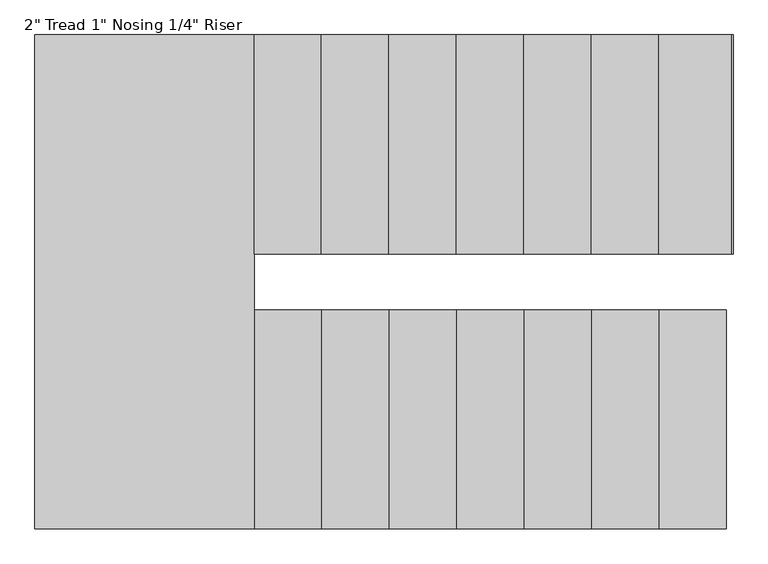
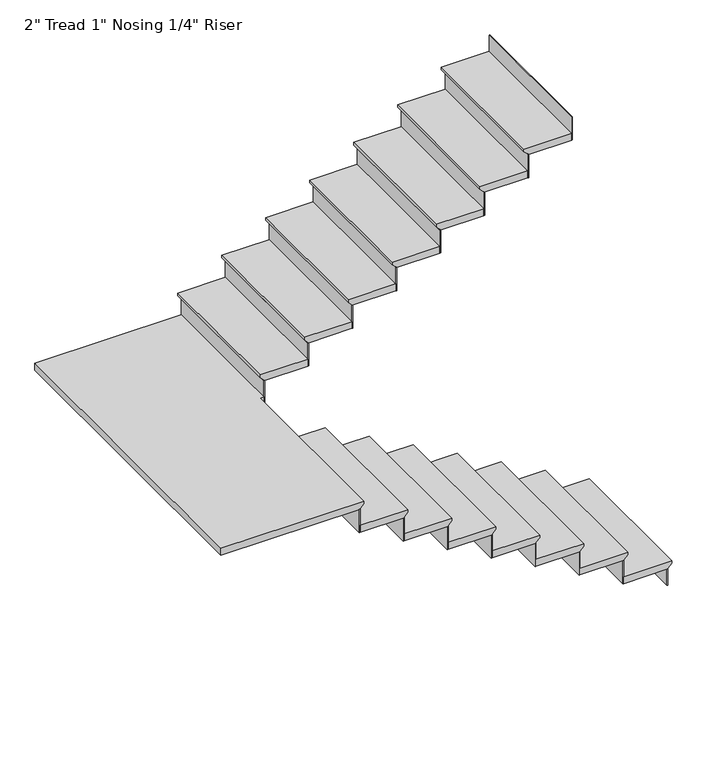
"""IFC4 building model written with IfcOpenShell, lengths in millimetres: stair flight geometry."""

from ifc_helpers import new_model, si_unit, origin, place, context, project, spatial, faceted_brep, source, transform, mapped, element, save


def stair_flight_128b20ea(model_context):
    return source(origin(), model_context, "Body", "Brep", [
        faceted_brep([(-11636.5023867, -1766.1499863, 3807.8833333), (-11636.5023867, -1766.1499863, 3826.9333333), (-11636.5023867, -2756.7499863, 3826.9333333), (-11636.5023867, -2756.7499863, 3807.8833333), (-11661.9023867, -1766.1499863, 3782.4833333), (-11661.9023867, -2756.7499863, 3782.4833333), (-11966.7023867, -1766.1499863, 3826.9333333), (-11966.7023867, -2756.7499863, 3826.9333333), (-11661.9023867, -2756.7499863, 3776.1333333), (-11966.7023867, -2756.7499863, 3776.1333333), (-11966.7023867, -1766.1499863, 3776.1333333), (-11661.9023867, -1766.1499863, 3776.1333333)], [[[0, 1, 2, 3]], [[4, 0, 3, 5]], [[2, 1, 6, 7]], [[8, 9, 10, 11]], [[2, 7, 9, 8, 5, 3]], [[8, 11, 4, 5]], [[6, 1, 0, 4, 11, 10]], [[7, 6, 10, 9]]]),
        faceted_brep([(-11661.9023867, -1766.1499863, 3776.1333333), (-11661.9023867, -1766.1499863, 3657.6), (-11668.2523867, -1766.1499863, 3657.6), (-11668.2523867, -1766.1499863, 3776.1333333), (-11661.9023867, -2756.7499863, 3776.1333333), (-11668.2523867, -2756.7499863, 3776.1333333), (-11668.2523867, -2756.7499863, 3657.6), (-11661.9023867, -2756.7499863, 3657.6)], [[[0, 1, 2, 3]], [[4, 5, 6, 7]], [[1, 0, 4, 7]], [[2, 1, 7, 6]], [[3, 2, 6, 5]], [[0, 3, 5, 4]]]),
        faceted_brep([(-11966.7023867, -1766.1499863, 3945.4666667), (-11966.7023867, -1766.1499863, 3776.1333333), (-11973.0523867, -1766.1499863, 3776.1333333), (-11973.0523867, -1766.1499863, 3945.4666667), (-11966.7023867, -2756.7499863, 3945.4666667), (-11973.0523867, -2756.7499863, 3945.4666667), (-11973.0523867, -2756.7499863, 3776.1333333), (-11966.7023867, -2756.7499863, 3776.1333333)], [[[0, 1, 2, 3]], [[4, 5, 6, 7]], [[1, 0, 4, 7]], [[2, 1, 7, 6]], [[3, 2, 6, 5]], [[0, 3, 5, 4]]]),
        faceted_brep([(-11941.3023867, -2756.7499863, 3996.2666667), (-11941.3023867, -1766.1499863, 3996.2666667), (-12271.5023867, -1766.1499863, 3996.2666667), (-12271.5023867, -2756.7499863, 3996.2666667), (-11966.7023867, -2756.7499863, 3945.4666667), (-12271.5023867, -2756.7499863, 3945.4666667), (-12271.5023867, -1766.1499863, 3945.4666667), (-11966.7023867, -1766.1499863, 3945.4666667), (-11966.7023867, -2756.7499863, 3951.8166667), (-11941.3023867, -2756.7499863, 3977.2166667), (-11966.7023867, -1766.1499863, 3951.8166667), (-11941.3023867, -1766.1499863, 3977.2166667)], [[[0, 1, 2, 3]], [[4, 5, 6, 7]], [[0, 3, 5, 4, 8, 9]], [[4, 7, 10, 8]], [[2, 1, 11, 10, 7, 6]], [[3, 2, 6, 5]], [[11, 1, 0, 9]], [[10, 11, 9, 8]]]),
        faceted_brep([(-12271.5023867, -1766.1499863, 4114.8), (-12271.5023867, -1766.1499863, 3945.4666667), (-12277.8523867, -1766.1499863, 3945.4666667), (-12277.8523867, -1766.1499863, 4114.8), (-12271.5023867, -2756.7499863, 4114.8), (-12277.8523867, -2756.7499863, 4114.8), (-12277.8523867, -2756.7499863, 3945.4666667), (-12271.5023867, -2756.7499863, 3945.4666667)], [[[0, 1, 2, 3]], [[4, 5, 6, 7]], [[1, 0, 4, 7]], [[2, 1, 7, 6]], [[3, 2, 6, 5]], [[0, 3, 5, 4]]]),
        faceted_brep([(-12246.1023867, -2756.7499863, 4165.6), (-12246.1023867, -1766.1499863, 4165.6), (-12576.3023867, -1766.1499863, 4165.6), (-12576.3023867, -2756.7499863, 4165.6), (-12271.5023867, -2756.7499863, 4114.8), (-12576.3023867, -2756.7499863, 4114.8), (-12576.3023867, -1766.1499863, 4114.8), (-12271.5023867, -1766.1499863, 4114.8), (-12271.5023867, -2756.7499863, 4121.15), (-12246.1023867, -2756.7499863, 4146.55), (-12271.5023867, -1766.1499863, 4121.15), (-12246.1023867, -1766.1499863, 4146.55)], [[[0, 1, 2, 3]], [[4, 5, 6, 7]], [[0, 3, 5, 4, 8, 9]], [[4, 7, 10, 8]], [[2, 1, 11, 10, 7, 6]], [[3, 2, 6, 5]], [[11, 1, 0, 9]], [[10, 11, 9, 8]]]),
        faceted_brep([(-12576.3023867, -1766.1499863, 4284.1333333), (-12576.3023867, -1766.1499863, 4114.8), (-12582.6523867, -1766.1499863, 4114.8), (-12582.6523867, -1766.1499863, 4284.1333333), (-12576.3023867, -2756.7499863, 4284.1333333), (-12582.6523867, -2756.7499863, 4284.1333333), (-12582.6523867, -2756.7499863, 4114.8), (-12576.3023867, -2756.7499863, 4114.8)], [[[0, 1, 2, 3]], [[4, 5, 6, 7]], [[1, 0, 4, 7]], [[2, 1, 7, 6]], [[3, 2, 6, 5]], [[0, 3, 5, 4]]]),
        faceted_brep([(-12550.9023867, -2756.7499863, 4334.9333333), (-12550.9023867, -1766.1499863, 4334.9333333), (-12881.1023867, -1766.1499863, 4334.9333333), (-12881.1023867, -2756.7499863, 4334.9333333), (-12576.3023867, -2756.7499863, 4284.1333333), (-12881.1023867, -2756.7499863, 4284.1333333), (-12881.1023867, -1766.1499863, 4284.1333333), (-12576.3023867, -1766.1499863, 4284.1333333), (-12576.3023867, -2756.7499863, 4290.4833333), (-12550.9023867, -2756.7499863, 4315.8833333), (-12576.3023867, -1766.1499863, 4290.4833333), (-12550.9023867, -1766.1499863, 4315.8833333)], [[[0, 1, 2, 3]], [[4, 5, 6, 7]], [[0, 3, 5, 4, 8, 9]], [[4, 7, 10, 8]], [[2, 1, 11, 10, 7, 6]], [[3, 2, 6, 5]], [[11, 1, 0, 9]], [[10, 11, 9, 8]]]),
        faceted_brep([(-12881.1023867, -1766.1499863, 4453.4666667), (-12881.1023867, -1766.1499863, 4284.1333333), (-12887.4523867, -1766.1499863, 4284.1333333), (-12887.4523867, -1766.1499863, 4453.4666667), (-12881.1023867, -2756.7499863, 4453.4666667), (-12887.4523867, -2756.7499863, 4453.4666667), (-12887.4523867, -2756.7499863, 4284.1333333), (-12881.1023867, -2756.7499863, 4284.1333333)], [[[0, 1, 2, 3]], [[4, 5, 6, 7]], [[1, 0, 4, 7]], [[2, 1, 7, 6]], [[3, 2, 6, 5]], [[0, 3, 5, 4]]]),
        faceted_brep([(-12855.7023867, -2756.7499863, 4504.2666667), (-12855.7023867, -1766.1499863, 4504.2666667), (-13185.9023867, -1766.1499863, 4504.2666667), (-13185.9023867, -2756.7499863, 4504.2666667), (-12881.1023867, -2756.7499863, 4453.4666667), (-13185.9023867, -2756.7499863, 4453.4666667), (-13185.9023867, -1766.1499863, 4453.4666667), (-12881.1023867, -1766.1499863, 4453.4666667), (-12881.1023867, -2756.7499863, 4459.8166667), (-12855.7023867, -2756.7499863, 4485.2166667), (-12881.1023867, -1766.1499863, 4459.8166667), (-12855.7023867, -1766.1499863, 4485.2166667)], [[[0, 1, 2, 3]], [[4, 5, 6, 7]], [[0, 3, 5, 4, 8, 9]], [[4, 7, 10, 8]], [[2, 1, 11, 10, 7, 6]], [[3, 2, 6, 5]], [[11, 1, 0, 9]], [[10, 11, 9, 8]]]),
        faceted_brep([(-13185.9023867, -1766.1499863, 4622.8), (-13185.9023867, -1766.1499863, 4453.4666667), (-13192.2523867, -1766.1499863, 4453.4666667), (-13192.2523867, -1766.1499863, 4622.8), (-13185.9023867, -2756.7499863, 4622.8), (-13192.2523867, -2756.7499863, 4622.8), (-13192.2523867, -2756.7499863, 4453.4666667), (-13185.9023867, -2756.7499863, 4453.4666667)], [[[0, 1, 2, 3]], [[4, 5, 6, 7]], [[1, 0, 4, 7]], [[2, 1, 7, 6]], [[3, 2, 6, 5]], [[0, 3, 5, 4]]]),
        faceted_brep([(-13160.5023867, -2756.7499863, 4673.6), (-13160.5023867, -1766.1499863, 4673.6), (-13490.7023867, -1766.1499863, 4673.6), (-13490.7023867, -2756.7499863, 4673.6), (-13185.9023867, -2756.7499863, 4622.8), (-13490.7023867, -2756.7499863, 4622.8), (-13490.7023867, -1766.1499863, 4622.8), (-13185.9023867, -1766.1499863, 4622.8), (-13185.9023867, -2756.7499863, 4629.15), (-13160.5023867, -2756.7499863, 4654.55), (-13185.9023867, -1766.1499863, 4629.15), (-13160.5023867, -1766.1499863, 4654.55)], [[[0, 1, 2, 3]], [[4, 5, 6, 7]], [[0, 3, 5, 4, 8, 9]], [[4, 7, 10, 8]], [[2, 1, 11, 10, 7, 6]], [[3, 2, 6, 5]], [[11, 1, 0, 9]], [[10, 11, 9, 8]]]),
        faceted_brep([(-13490.7023867, -1766.1499863, 4792.1333333), (-13490.7023867, -1766.1499863, 4622.8), (-13497.0523867, -1766.1499863, 4622.8), (-13497.0523867, -1766.1499863, 4792.1333333), (-13490.7023867, -2756.7499863, 4792.1333333), (-13497.0523867, -2756.7499863, 4792.1333333), (-13497.0523867, -2756.7499863, 4622.8), (-13490.7023867, -2756.7499863, 4622.8)], [[[0, 1, 2, 3]], [[4, 5, 6, 7]], [[1, 0, 4, 7]], [[2, 1, 7, 6]], [[3, 2, 6, 5]], [[0, 3, 5, 4]]]),
        faceted_brep([(-13465.3023867, -2756.7499863, 4842.9333333), (-13465.3023867, -1766.1499863, 4842.9333333), (-13795.5023867, -1766.1499863, 4842.9333333), (-13795.5023867, -2756.7499863, 4842.9333333), (-13490.7023867, -2756.7499863, 4792.1333333), (-13795.5023867, -2756.7499863, 4792.1333333), (-13795.5023867, -1766.1499863, 4792.1333333), (-13490.7023867, -1766.1499863, 4792.1333333), (-13490.7023867, -2756.7499863, 4798.4833333), (-13465.3023867, -2756.7499863, 4823.8833333), (-13490.7023867, -1766.1499863, 4798.4833333), (-13465.3023867, -1766.1499863, 4823.8833333)], [[[0, 1, 2, 3]], [[4, 5, 6, 7]], [[0, 3, 5, 4, 8, 9]], [[4, 7, 10, 8]], [[2, 1, 11, 10, 7, 6]], [[3, 2, 6, 5]], [[11, 1, 0, 9]], [[10, 11, 9, 8]]]),
        faceted_brep([(-13795.5023867, -1766.1499863, 4961.4666667), (-13795.5023867, -1766.1499863, 4792.1333333), (-13801.8523867, -1766.1499863, 4792.1333333), (-13801.8523867, -1766.1499863, 4961.4666667), (-13795.5023867, -2756.7499863, 4961.4666667), (-13801.8523867, -2756.7499863, 4961.4666667), (-13801.8523867, -2756.7499863, 4792.1333333), (-13795.5023867, -2756.7499863, 4792.1333333)], [[[0, 1, 2, 3]], [[4, 5, 6, 7]], [[1, 0, 4, 7]], [[2, 1, 7, 6]], [[3, 2, 6, 5]], [[0, 3, 5, 4]]]),
        faceted_brep([(-13744.7023867, -521.5499863, 5012.2666667), (-14760.7023867, -521.5499863, 5012.2666667), (-14760.7023867, -2756.7499863, 5012.2666667), (-13770.1023867, -2756.7499863, 5012.2666667), (-13770.1023867, -1512.1499863, 5012.2666667), (-13744.7023867, -1512.1499863, 5012.2666667), (-14760.7023867, -521.5499863, 4961.4666667), (-13744.7023867, -521.5499863, 4961.4666667), (-13744.7023867, -1512.1499863, 4961.4666667), (-13770.1023867, -1512.1499863, 4961.4666667), (-13770.1023867, -1766.1499863, 4961.4666667), (-13795.5023867, -1766.1499863, 4961.4666667), (-13795.5023867, -2756.7499863, 4961.4666667), (-14760.7023867, -2756.7499863, 4961.4666667), (-13795.5023867, -2756.7499863, 4967.8166667), (-13770.1023867, -2756.7499863, 4993.2166667), (-13795.5023867, -1766.1499863, 4967.8166667), (-13770.1023867, -1766.1499863, 4993.2166667)], [[[0, 1, 2, 3, 4, 5]], [[6, 7, 8, 9, 10, 11, 12, 13]], [[1, 0, 7, 6]], [[2, 1, 6, 13]], [[3, 2, 13, 12, 14, 15]], [[12, 11, 16, 14]], [[11, 10, 17, 16]], [[4, 3, 15, 17, 10, 9]], [[5, 4, 9, 8]], [[0, 5, 8, 7]], [[15, 14, 16, 17]]]),
        faceted_brep([(-13744.7023867, -1512.1499863, 5130.8), (-13744.7023867, -1512.1499863, 4961.4666667), (-13738.3523867, -1512.1499863, 4961.4666667), (-13738.3523867, -1512.1499863, 5130.8), (-13744.7023867, -521.5499863, 5130.8), (-13738.3523867, -521.5499863, 5130.8), (-13738.3523867, -521.5499863, 4961.4666667), (-13744.7023867, -521.5499863, 4961.4666667)], [[[0, 1, 2, 3]], [[4, 5, 6, 7]], [[1, 0, 4, 7]], [[2, 1, 7, 6]], [[3, 2, 6, 5]], [[0, 3, 5, 4]]]),
        faceted_brep([(-13770.1023867, -521.5499863, 5181.6), (-13770.1023867, -1512.1499863, 5181.6), (-13439.9023867, -1512.1499863, 5181.6), (-13439.9023867, -521.5499863, 5181.6), (-13744.7023867, -521.5499863, 5130.8), (-13439.9023867, -521.5499863, 5130.8), (-13439.9023867, -1512.1499863, 5130.8), (-13744.7023867, -1512.1499863, 5130.8), (-13744.7023867, -521.5499863, 5137.15), (-13770.1023867, -521.5499863, 5162.55), (-13744.7023867, -1512.1499863, 5137.15), (-13770.1023867, -1512.1499863, 5162.55)], [[[0, 1, 2, 3]], [[4, 5, 6, 7]], [[0, 3, 5, 4, 8, 9]], [[4, 7, 10, 8]], [[2, 1, 11, 10, 7, 6]], [[3, 2, 6, 5]], [[11, 1, 0, 9]], [[10, 11, 9, 8]]]),
        faceted_brep([(-13439.9023867, -1512.1499863, 5300.1333333), (-13439.9023867, -1512.1499863, 5130.8), (-13433.5523867, -1512.1499863, 5130.8), (-13433.5523867, -1512.1499863, 5300.1333333), (-13439.9023867, -521.5499863, 5300.1333333), (-13433.5523867, -521.5499863, 5300.1333333), (-13433.5523867, -521.5499863, 5130.8), (-13439.9023867, -521.5499863, 5130.8)], [[[0, 1, 2, 3]], [[4, 5, 6, 7]], [[1, 0, 4, 7]], [[2, 1, 7, 6]], [[3, 2, 6, 5]], [[0, 3, 5, 4]]]),
        faceted_brep([(-13465.3023867, -521.5499863, 5350.9333333), (-13465.3023867, -1512.1499863, 5350.9333333), (-13135.1023867, -1512.1499863, 5350.9333333), (-13135.1023867, -521.5499863, 5350.9333333), (-13439.9023867, -521.5499863, 5300.1333333), (-13135.1023867, -521.5499863, 5300.1333333), (-13135.1023867, -1512.1499863, 5300.1333333), (-13439.9023867, -1512.1499863, 5300.1333333), (-13439.9023867, -521.5499863, 5306.4833333), (-13465.3023867, -521.5499863, 5331.8833333), (-13439.9023867, -1512.1499863, 5306.4833333), (-13465.3023867, -1512.1499863, 5331.8833333)], [[[0, 1, 2, 3]], [[4, 5, 6, 7]], [[0, 3, 5, 4, 8, 9]], [[4, 7, 10, 8]], [[2, 1, 11, 10, 7, 6]], [[3, 2, 6, 5]], [[11, 1, 0, 9]], [[10, 11, 9, 8]]]),
        faceted_brep([(-13135.1023867, -1512.1499863, 5469.4666667), (-13135.1023867, -1512.1499863, 5300.1333333), (-13128.7523867, -1512.1499863, 5300.1333333), (-13128.7523867, -1512.1499863, 5469.4666667), (-13135.1023867, -521.5499863, 5469.4666667), (-13128.7523867, -521.5499863, 5469.4666667), (-13128.7523867, -521.5499863, 5300.1333333), (-13135.1023867, -521.5499863, 5300.1333333)], [[[0, 1, 2, 3]], [[4, 5, 6, 7]], [[1, 0, 4, 7]], [[2, 1, 7, 6]], [[3, 2, 6, 5]], [[0, 3, 5, 4]]]),
        faceted_brep([(-13160.5023867, -521.5499863, 5520.2666667), (-13160.5023867, -1512.1499863, 5520.2666667), (-12830.3023867, -1512.1499863, 5520.2666667), (-12830.3023867, -521.5499863, 5520.2666667), (-13135.1023867, -521.5499863, 5469.4666667), (-12830.3023867, -521.5499863, 5469.4666667), (-12830.3023867, -1512.1499863, 5469.4666667), (-13135.1023867, -1512.1499863, 5469.4666667), (-13135.1023867, -521.5499863, 5475.8166667), (-13160.5023867, -521.5499863, 5501.2166667), (-13135.1023867, -1512.1499863, 5475.8166667), (-13160.5023867, -1512.1499863, 5501.2166667)], [[[0, 1, 2, 3]], [[4, 5, 6, 7]], [[0, 3, 5, 4, 8, 9]], [[4, 7, 10, 8]], [[2, 1, 11, 10, 7, 6]], [[3, 2, 6, 5]], [[11, 1, 0, 9]], [[10, 11, 9, 8]]]),
        faceted_brep([(-12830.3023867, -1512.1499863, 5638.8), (-12830.3023867, -1512.1499863, 5469.4666667), (-12823.9523867, -1512.1499863, 5469.4666667), (-12823.9523867, -1512.1499863, 5638.8), (-12830.3023867, -521.5499863, 5638.8), (-12823.9523867, -521.5499863, 5638.8), (-12823.9523867, -521.5499863, 5469.4666667), (-12830.3023867, -521.5499863, 5469.4666667)], [[[0, 1, 2, 3]], [[4, 5, 6, 7]], [[1, 0, 4, 7]], [[2, 1, 7, 6]], [[3, 2, 6, 5]], [[0, 3, 5, 4]]]),
        faceted_brep([(-12855.7023867, -521.5499863, 5689.6), (-12855.7023867, -1512.1499863, 5689.6), (-12525.5023867, -1512.1499863, 5689.6), (-12525.5023867, -521.5499863, 5689.6), (-12830.3023867, -521.5499863, 5638.8), (-12525.5023867, -521.5499863, 5638.8), (-12525.5023867, -1512.1499863, 5638.8), (-12830.3023867, -1512.1499863, 5638.8), (-12830.3023867, -521.5499863, 5645.15), (-12855.7023867, -521.5499863, 5670.55), (-12830.3023867, -1512.1499863, 5645.15), (-12855.7023867, -1512.1499863, 5670.55)], [[[0, 1, 2, 3]], [[4, 5, 6, 7]], [[0, 3, 5, 4, 8, 9]], [[4, 7, 10, 8]], [[2, 1, 11, 10, 7, 6]], [[3, 2, 6, 5]], [[11, 1, 0, 9]], [[10, 11, 9, 8]]]),
        faceted_brep([(-12525.5023867, -1512.1499863, 5808.1333333), (-12525.5023867, -1512.1499863, 5638.8), (-12519.1523867, -1512.1499863, 5638.8), (-12519.1523867, -1512.1499863, 5808.1333333), (-12525.5023867, -521.5499863, 5808.1333333), (-12519.1523867, -521.5499863, 5808.1333333), (-12519.1523867, -521.5499863, 5638.8), (-12525.5023867, -521.5499863, 5638.8)], [[[0, 1, 2, 3]], [[4, 5, 6, 7]], [[1, 0, 4, 7]], [[2, 1, 7, 6]], [[3, 2, 6, 5]], [[0, 3, 5, 4]]]),
        faceted_brep([(-12550.9023867, -521.5499863, 5858.9333333), (-12550.9023867, -1512.1499863, 5858.9333333), (-12220.7023867, -1512.1499863, 5858.9333333), (-12220.7023867, -521.5499863, 5858.9333333), (-12525.5023867, -521.5499863, 5808.1333333), (-12220.7023867, -521.5499863, 5808.1333333), (-12220.7023867, -1512.1499863, 5808.1333333), (-12525.5023867, -1512.1499863, 5808.1333333), (-12525.5023867, -521.5499863, 5814.4833333), (-12550.9023867, -521.5499863, 5839.8833333), (-12525.5023867, -1512.1499863, 5814.4833333), (-12550.9023867, -1512.1499863, 5839.8833333)], [[[0, 1, 2, 3]], [[4, 5, 6, 7]], [[0, 3, 5, 4, 8, 9]], [[4, 7, 10, 8]], [[2, 1, 11, 10, 7, 6]], [[3, 2, 6, 5]], [[11, 1, 0, 9]], [[10, 11, 9, 8]]]),
        faceted_brep([(-12220.7023867, -1512.1499863, 5977.4666667), (-12220.7023867, -1512.1499863, 5808.1333333), (-12214.3523867, -1512.1499863, 5808.1333333), (-12214.3523867, -1512.1499863, 5977.4666667), (-12220.7023867, -521.5499863, 5977.4666667), (-12214.3523867, -521.5499863, 5977.4666667), (-12214.3523867, -521.5499863, 5808.1333333), (-12220.7023867, -521.5499863, 5808.1333333)], [[[0, 1, 2, 3]], [[4, 5, 6, 7]], [[1, 0, 4, 7]], [[2, 1, 7, 6]], [[3, 2, 6, 5]], [[0, 3, 5, 4]]]),
        faceted_brep([(-12246.1023867, -521.5499863, 6028.2666667), (-12246.1023867, -1512.1499863, 6028.2666667), (-11915.9023867, -1512.1499863, 6028.2666667), (-11915.9023867, -521.5499863, 6028.2666667), (-12220.7023867, -521.5499863, 5977.4666667), (-11915.9023867, -521.5499863, 5977.4666667), (-11915.9023867, -1512.1499863, 5977.4666667), (-12220.7023867, -1512.1499863, 5977.4666667), (-12220.7023867, -521.5499863, 5983.8166667), (-12246.1023867, -521.5499863, 6009.2166667), (-12220.7023867, -1512.1499863, 5983.8166667), (-12246.1023867, -1512.1499863, 6009.2166667)], [[[0, 1, 2, 3]], [[4, 5, 6, 7]], [[0, 3, 5, 4, 8, 9]], [[4, 7, 10, 8]], [[2, 1, 11, 10, 7, 6]], [[3, 2, 6, 5]], [[11, 1, 0, 9]], [[10, 11, 9, 8]]]),
        faceted_brep([(-11915.9023867, -1512.1499863, 6146.8), (-11915.9023867, -1512.1499863, 5977.4666667), (-11909.5523867, -1512.1499863, 5977.4666667), (-11909.5523867, -1512.1499863, 6146.8), (-11915.9023867, -521.5499863, 6146.8), (-11909.5523867, -521.5499863, 6146.8), (-11909.5523867, -521.5499863, 5977.4666667), (-11915.9023867, -521.5499863, 5977.4666667)], [[[0, 1, 2, 3]], [[4, 5, 6, 7]], [[1, 0, 4, 7]], [[2, 1, 7, 6]], [[3, 2, 6, 5]], [[0, 3, 5, 4]]]),
        faceted_brep([(-11611.1023867, -1512.1499863, 6316.1333333), (-11611.1023867, -1512.1499863, 6146.8), (-11604.7523867, -1512.1499863, 6146.8), (-11604.7523867, -1512.1499863, 6316.1333333), (-11611.1023867, -521.5499863, 6316.1333333), (-11604.7523867, -521.5499863, 6316.1333333), (-11604.7523867, -521.5499863, 6146.8), (-11611.1023867, -521.5499863, 6146.8)], [[[0, 1, 2, 3]], [[4, 5, 6, 7]], [[1, 0, 4, 7]], [[2, 1, 7, 6]], [[3, 2, 6, 5]], [[0, 3, 5, 4]]]),
        faceted_brep([(-11941.3023867, -521.5499863, 6197.6), (-11941.3023867, -1512.1499863, 6197.6), (-11611.1023867, -1512.1499863, 6197.6), (-11611.1023867, -521.5499863, 6197.6), (-11915.9023867, -521.5499863, 6146.8), (-11611.1023867, -521.5499863, 6146.8), (-11611.1023867, -1512.1499863, 6146.8), (-11915.9023867, -1512.1499863, 6146.8), (-11915.9023867, -521.5499863, 6153.15), (-11941.3023867, -521.5499863, 6178.55), (-11915.9023867, -1512.1499863, 6153.15), (-11941.3023867, -1512.1499863, 6178.55)], [[[0, 1, 2, 3]], [[4, 5, 6, 7]], [[0, 3, 5, 4, 8, 9]], [[4, 7, 10, 8]], [[2, 1, 11, 10, 7, 6]], [[3, 2, 6, 5]], [[11, 1, 0, 9]], [[10, 11, 9, 8]]]),
    ])


if __name__ == "__main__":
    model = new_model("IFC4")
    model_context = context("Model", 3, world=origin())
    ifc_project = project(units=[si_unit("LENGTHUNIT", "METRE", prefix="MILLI")], contexts=[model_context])
    site = spatial("IfcSite", under=ifc_project)
    building = spatial("IfcBuilding", under=site)
    placement = place(None, origin())
    stair_flight_shape = stair_flight_128b20ea(model_context)
    element("IfcStairFlight", 1, ObjectType="2\" Tread 1\" Nosing 1/4\" Riser", at=placement, inside=building, context=model_context, shape_type="MappedRepresentation", body=[
        mapped(stair_flight_shape, transform((0.0, 0.0, 0.0), x_axis=(1.0, 0.0, 0.0), y_axis=(0.0, 1.0, 0.0), z_axis=(0.0, 0.0, 1.0))),
    ])
    save(model, "model.ifc")
